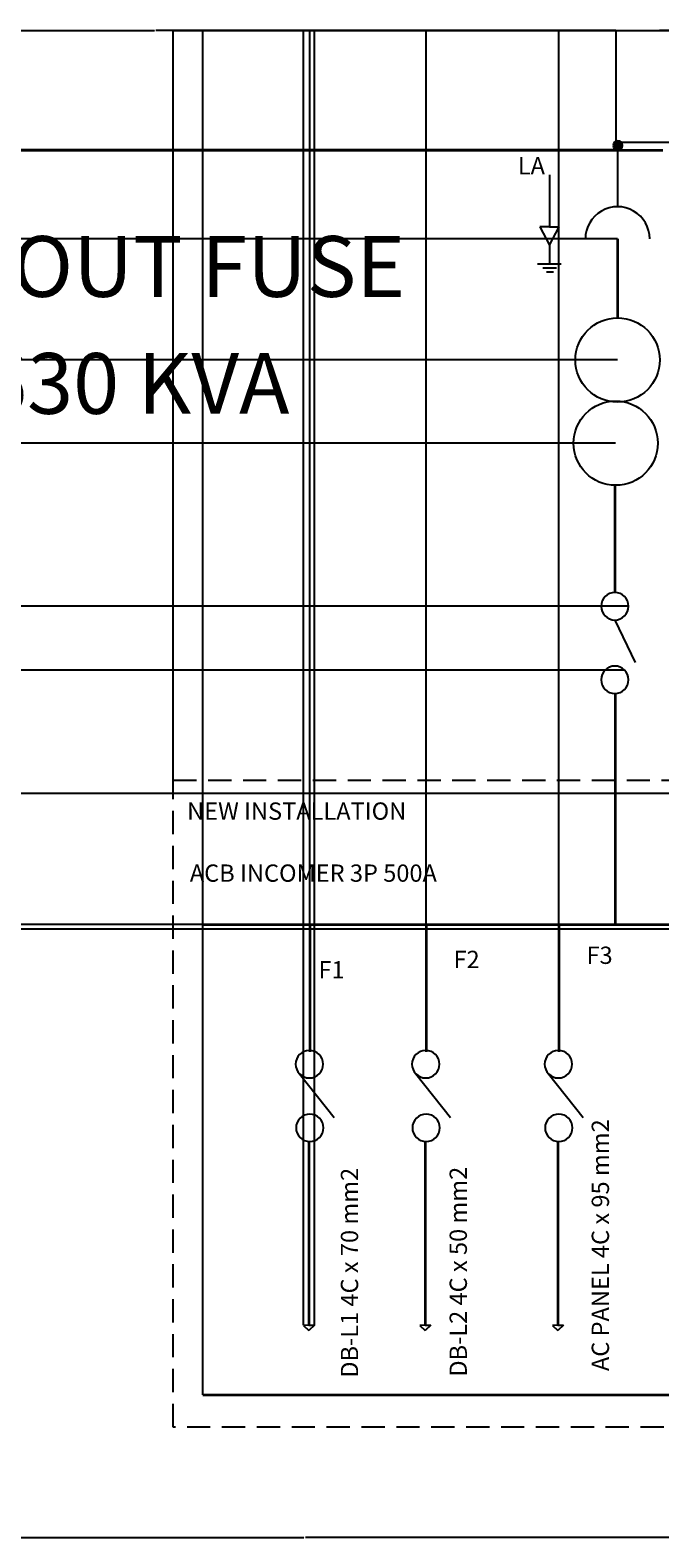
# Model space of a CAD drawing. Units: millimetres. Extents: x 1832 to 3146, y 927 to 1751.
# Tile 3 of 4: x 2339 to 2683, y 927 to 1751. Entities that reach past the tile are written whole.
import ezdxf

# ---------------------------------------------------------------- set-up
doc = ezdxf.new("R2010")
doc.units = ezdxf.units.MM
doc.header["$MEASUREMENT"] = 0
doc.linetypes.add('DASHED', pattern=[19.05, 12.7, -6.35])
doc.layers.get('0').update_dxf_attribs({"color": 2, "lineweight": 35})
doc.layers.get('0').transparency = 0.01
for name, color, linetype, lineweight in [('A-ANNO-DIMS', 2, 'Continuous', 18), ('E-ANNO-TEXT', 7, 'Continuous', 18), ('E-POWR-EQPM', 2, 'Continuous', 25), ('E-POWR-PNLS', 3, 'DASHED', 25), ('E-POWR-WIRE', 7, 'Continuous', 35)]:
    doc.layers.add(name, color=color, linetype=linetype, lineweight=lineweight)
doc.styles.get("Standard").update_dxf_attribs({"font": 'arial.ttf'})
doc.dimstyles.get("Standard").update_dxf_attribs({"dimtxt": 0.18, "dimasz": 0.18, "dimexe": 0.18, "dimexo": 0.0625, "dimgap": 0.09, "dimtad": 0, "dimtih": 1, "dimtoh": 1, "dimdec": 4, "dimzin": 0, "dimdsep": 46, "dimtxsty": 'Standard', "dimcen": 0.09, "dimadec": 0, "dimazin": 0, "dimtfac": 1, "dimtdec": 4, "dimtofl": 0, "dimtmove": 0, "dimatfit": 3, "dimfxl": 1, "dimtolj": 1, "dimtzin": 0, "dimarcsym": 0})

# ---------------------------------------------------------------- blocks, each defined once
blk = doc.blocks.new('CB-FEEDER')
blk.add_line((1982.97, 1178.23), (2001.83, 1154.39))
for points in [[(1980.83, 1183.48, 1), (1995.83, 1183.48, 1)], [(1981.05, 1148.75, 1), (1996.05, 1148.75, 1)]]:
    blk.add_lwpolyline(points, format="xyb", close=True)
blk = doc.blocks.new('CB-INCOMER')
blk.add_line((2155.16, 1426.14), (2166.26, 1402.88))
for points in [[(2147.67, 1433.64, 1), (2162.67, 1433.64, 1)], [(2147.67, 1393.5, 1), (2162.67, 1393.5, 1)]]:
    blk.add_lwpolyline(points, format="xyb", close=True)
blk = doc.blocks.new('CABLE-ARROW')
for p, q in [((1988.1, 1040.89), (1985.1, 1040.84)), ((1985.1, 1040.84), (1988.1, 1038.05)), ((1988.1, 1040.89), (1991.1, 1040.89)), ((1991.1, 1040.89), (1988.1, 1038.05))]:
    blk.add_line(p, q)
blk = doc.blocks.new('LIGHTNING-ARRESTER')
for p, q in [((2119.54, 1669.38), (2119.54, 1640.82)), ((2119.54, 1640.82), (2114.27, 1640.82)), ((2114.27, 1640.82), (2119.54, 1630.9)), ((2119.54, 1640.82), (2124.8, 1640.82)), ((2119.54, 1630.9), (2124.8, 1640.82)), ((2119.54, 1630.9), (2119.54, 1620.77)), ((2112.86, 1620.77), (2125.9, 1620.77)), ((2115.79, 1618.51), (2123.28, 1618.51)), ((2117.89, 1616.41), (2121.66, 1616.41))]:
    blk.add_line(p, q)
blk = doc.blocks.new('DROPOUT-FUSE')
h = blk.add_hatch(color=256)
h.dxf.hatch_style = 1
h.paths.add_polyline_path([(2154.3, 1685.32), (2159.3, 1685.32, 1)])
h.paths.add_polyline_path([(2159.3, 1685.32), (2154.3, 1685.32, 1)])
blk.add_line((2156.63, 1682.82), (2156.63, 1651.9))
blk.add_lwpolyline([(2154.3, 1685.32, 1), (2159.3, 1685.32, 1)], format="xyb", close=True)
blk.add_arc((2156.63, 1634.33), 17.57, 359.97103, 180.02897)
blk = doc.blocks.new('TRANSFORMER')
for centre in [(2156.63, 1568.17), (2155.63, 1522.72)]:
    blk.add_circle(centre, 23.01)
blk = doc.blocks.new('*D9')
at = {"layer": 'A-ANNO-DIMS', "color": 0, "lineweight": -2, "transparency": 16777216}
for p, q in [((1892.94, 1002.86), (1892.94, 927.26)), ((3085.33, 987.73), (3085.33, 927.26)), ((1893.12, 927.44), (2488.68, 927.44)), ((3085.15, 927.44), (2489.59, 927.44))]:
    blk.add_line(p, q, dxfattribs=at)
at = {"layer": 'A-ANNO-DIMS', "color": 0, "lineweight": 35, "transparency": 16777216}
for points in [[(1893.12, 927.47), (1893.12, 927.41), (1892.94, 927.44)], [(3085.15, 927.47), (3085.15, 927.41), (3085.33, 927.44)]]:
    blk.add_solid(points, dxfattribs=at)
at = {"layer": 'Defpoints', "color": 0, "lineweight": 35, "transparency": 16777216}
for p in [(1892.94, 1002.93), (3085.33, 987.79), (3085.33, 927.44)]:
    blk.add_point(p, dxfattribs=at)
at = {"layer": 'A-ANNO-DIMS', "color": 0, "transparency": 16777216, "insert": (2489.13, 927.44), "char_height": 0.18, "attachment_point": 5}
blk.add_mtext('\\A1;1192.4', dxfattribs=at)
blk = doc.blocks.new('*D10')
at = {"layer": 'A-ANNO-DIMS', "color": 0, "lineweight": -2, "transparency": 16777216}
for p, q in [((2658.48, 1689.58), (3145.86, 1689.58)), ((3145.68, 1689.4), (3145.68, 1338.87)), ((3145.68, 987.97), (3145.68, 1338.5)), ((3085.39, 987.79), (3145.86, 987.79))]:
    blk.add_line(p, q, dxfattribs=at)
at = {"layer": 'A-ANNO-DIMS', "color": 0, "lineweight": 35, "transparency": 16777216}
for points in [[(3145.65, 1689.4), (3145.71, 1689.4), (3145.68, 1689.58)], [(3145.65, 987.97), (3145.71, 987.97), (3145.68, 987.79)]]:
    blk.add_solid(points, dxfattribs=at)
at = {"layer": 'Defpoints', "color": 0, "lineweight": 35, "transparency": 16777216}
for p in [(2658.42, 1689.58), (3145.68, 1689.58), (3085.33, 987.79)]:
    blk.add_point(p, dxfattribs=at)
at = {"layer": 'A-ANNO-DIMS', "color": 0, "transparency": 16777216, "insert": (3145.68, 1338.68), "char_height": 0.18, "attachment_point": 5}
blk.add_mtext('\\A1;701.8', dxfattribs=at)
blk = doc.blocks.new('*D16')
at = {"layer": 'A-ANNO-DIMS', "color": 0, "lineweight": -2, "transparency": 16777216}
for p, q in [((2491.94, 1262.43), (2491.94, 1750.84)), ((2492.12, 1750.66), (2523.31, 1750.66)), ((2555.29, 1750.66), (2524.1, 1750.66)), ((2555.47, 1262.43), (2555.47, 1750.84))]:
    blk.add_line(p, q, dxfattribs=at)
at = {"layer": 'A-ANNO-DIMS', "color": 0, "lineweight": 35, "transparency": 16777216}
for points in [[(2492.12, 1750.69), (2492.12, 1750.63), (2491.94, 1750.66)], [(2555.29, 1750.69), (2555.29, 1750.63), (2555.47, 1750.66)]]:
    blk.add_solid(points, dxfattribs=at)
at = {"layer": 'Defpoints', "color": 0, "lineweight": 35, "transparency": 16777216}
for p in [(2555.47, 1750.66), (2491.94, 1262.37), (2555.47, 1262.37)]:
    blk.add_point(p, dxfattribs=at)
at = {"layer": 'A-ANNO-DIMS', "color": 0, "transparency": 16777216, "insert": (2523.7, 1750.66), "char_height": 0.18, "attachment_point": 5}
blk.add_mtext('\\A1;63.53', dxfattribs=at)
blk = doc.blocks.new('*D17')
at = {"layer": 'A-ANNO-DIMS', "color": 0, "lineweight": -2, "transparency": 16777216}
for p, q in [((2555.47, 1262.43), (2555.47, 1750.84)), ((2555.65, 1750.66), (2591.3, 1750.66)), ((2627.74, 1750.66), (2592.09, 1750.66)), ((2627.92, 1262.43), (2627.92, 1750.84))]:
    blk.add_line(p, q, dxfattribs=at)
at = {"layer": 'A-ANNO-DIMS', "color": 0, "lineweight": 35, "transparency": 16777216}
for points in [[(2555.65, 1750.69), (2555.65, 1750.63), (2555.47, 1750.66)], [(2627.74, 1750.69), (2627.74, 1750.63), (2627.92, 1750.66)]]:
    blk.add_solid(points, dxfattribs=at)
at = {"layer": 'Defpoints', "color": 0, "lineweight": 35, "transparency": 16777216}
for p in [(2627.92, 1750.66), (2555.47, 1262.37), (2627.92, 1262.37)]:
    blk.add_point(p, dxfattribs=at)
at = {"layer": 'A-ANNO-DIMS', "color": 0, "transparency": 16777216, "insert": (2591.69, 1750.66), "char_height": 0.18, "attachment_point": 5}
blk.add_mtext('\\A1;72.45', dxfattribs=at)
blk = doc.blocks.new('*D18')
at = {"layer": 'A-ANNO-DIMS', "color": 0, "lineweight": -2, "transparency": 16777216}
for p, q in [((2627.92, 1262.43), (2627.92, 1750.84)), ((2628.1, 1750.66), (2682.1, 1750.66)), ((2737.01, 1750.66), (2683.01, 1750.66)), ((2737.19, 1262.43), (2737.19, 1750.84))]:
    blk.add_line(p, q, dxfattribs=at)
at = {"layer": 'A-ANNO-DIMS', "color": 0, "lineweight": 35, "transparency": 16777216}
for points in [[(2628.1, 1750.69), (2628.1, 1750.63), (2627.92, 1750.66)], [(2737.01, 1750.69), (2737.01, 1750.63), (2737.19, 1750.66)]]:
    blk.add_solid(points, dxfattribs=at)
at = {"layer": 'Defpoints', "color": 0, "lineweight": 35, "transparency": 16777216}
for p in [(2737.19, 1750.66), (2627.92, 1262.37), (2737.19, 1262.37)]:
    blk.add_point(p, dxfattribs=at)
at = {"layer": 'A-ANNO-DIMS', "color": 0, "transparency": 16777216, "insert": (2682.56, 1750.66), "char_height": 0.18, "attachment_point": 5}
blk.add_mtext('\\A1;109.27', dxfattribs=at)
blk = doc.blocks.new('*D21')
at = {"layer": 'A-ANNO-DIMS', "color": 0, "lineweight": -2, "transparency": 16777216}
for p, q in [((2155.83, 1687.68), (2155.83, 1750.84)), ((2156.01, 1750.66), (2407.13, 1750.66)), ((2659.03, 1750.66), (2407.91, 1750.66)), ((2659.21, 1690.18), (2659.21, 1750.84))]:
    blk.add_line(p, q, dxfattribs=at)
at = {"layer": 'A-ANNO-DIMS', "color": 0, "lineweight": 35, "transparency": 16777216}
for points in [[(2156.01, 1750.69), (2156.01, 1750.63), (2155.83, 1750.66)], [(2659.03, 1750.69), (2659.03, 1750.63), (2659.21, 1750.66)]]:
    blk.add_solid(points, dxfattribs=at)
at = {"layer": 'Defpoints', "color": 0, "lineweight": 35, "transparency": 16777216}
for p in [(2659.21, 1750.66), (2659.21, 1690.11), (2155.83, 1687.62)]:
    blk.add_point(p, dxfattribs=at)
at = {"layer": 'A-ANNO-DIMS', "color": 0, "transparency": 16777216, "insert": (2407.52, 1750.66), "char_height": 0.18, "attachment_point": 5}
blk.add_mtext('\\A1;503.4', dxfattribs=at)
blk = doc.blocks.new('*D26')
at = {"layer": 'A-ANNO-DIMS', "color": 0, "lineweight": -2, "transparency": 16777216}
for p, q in [((2417.38, 1341.25), (2417.38, 1750.84)), ((2417.56, 1750.66), (2750.89, 1750.66)), ((3085.15, 1750.66), (2751.82, 1750.66)), ((3085.33, 1341.25), (3085.33, 1750.84))]:
    blk.add_line(p, q, dxfattribs=at)
at = {"layer": 'A-ANNO-DIMS', "color": 0, "lineweight": 35, "transparency": 16777216}
for points in [[(2417.56, 1750.69), (2417.56, 1750.63), (2417.38, 1750.66)], [(3085.15, 1750.69), (3085.15, 1750.63), (3085.33, 1750.66)]]:
    blk.add_solid(points, dxfattribs=at)
at = {"layer": 'Defpoints', "color": 0, "lineweight": 35, "transparency": 16777216}
for p in [(3085.33, 1750.66), (2417.38, 1341.19), (3085.33, 1341.19)]:
    blk.add_point(p, dxfattribs=at)
at = {"layer": 'A-ANNO-DIMS', "color": 0, "transparency": 16777216, "insert": (2751.35, 1750.66), "char_height": 0.18, "attachment_point": 5}
blk.add_mtext('\\A1;667.94', dxfattribs=at)
blk = doc.blocks.new('*D28')
at = {"layer": 'A-ANNO-DIMS', "color": 0, "lineweight": -2, "transparency": 16777216}
for p, q in [((2433.56, 1005.45), (2433.56, 1750.84)), ((2433.74, 1750.66), (2748.28, 1750.66)), ((3063.74, 1750.66), (2749.21, 1750.66)), ((3063.92, 1005.45), (3063.92, 1750.84))]:
    blk.add_line(p, q, dxfattribs=at)
at = {"layer": 'A-ANNO-DIMS', "color": 0, "lineweight": 35, "transparency": 16777216}
for points in [[(2433.74, 1750.69), (2433.74, 1750.63), (2433.56, 1750.66)], [(3063.74, 1750.69), (3063.74, 1750.63), (3063.92, 1750.66)]]:
    blk.add_solid(points, dxfattribs=at)
at = {"layer": 'Defpoints', "color": 0, "lineweight": 35, "transparency": 16777216}
for p in [(3063.92, 1750.66), (2433.56, 1005.39), (3063.92, 1005.39)]:
    blk.add_point(p, dxfattribs=at)
at = {"layer": 'A-ANNO-DIMS', "color": 0, "transparency": 16777216, "insert": (2748.74, 1750.66), "char_height": 0.18, "attachment_point": 5}
blk.add_mtext('\\A1;630.36', dxfattribs=at)
blk = doc.blocks.new('*D30')
at = {"layer": 'A-ANNO-DIMS', "color": 0, "lineweight": -2, "transparency": 16777216}
for p, q in [((2433.56, 1262.43), (2433.56, 1750.84)), ((2433.74, 1750.66), (2462.36, 1750.66)), ((2491.76, 1750.66), (2463.14, 1750.66)), ((2491.94, 1262.43), (2491.94, 1750.84))]:
    blk.add_line(p, q, dxfattribs=at)
at = {"layer": 'A-ANNO-DIMS', "color": 0, "lineweight": 35, "transparency": 16777216}
for points in [[(2433.74, 1750.69), (2433.74, 1750.63), (2433.56, 1750.66)], [(2491.76, 1750.69), (2491.76, 1750.63), (2491.94, 1750.66)]]:
    blk.add_solid(points, dxfattribs=at)
at = {"layer": 'Defpoints', "color": 0, "lineweight": 35, "transparency": 16777216}
for p in [(2491.94, 1750.66), (2433.56, 1262.37), (2491.94, 1262.37)]:
    blk.add_point(p, dxfattribs=at)
at = {"layer": 'A-ANNO-DIMS', "color": 0, "transparency": 16777216, "insert": (2462.75, 1750.66), "char_height": 0.18, "attachment_point": 5}
blk.add_mtext('\\A1;58.37', dxfattribs=at)
blk = doc.blocks.new('*D33')
at = {"layer": 'A-ANNO-DIMS', "color": 0, "lineweight": -2, "transparency": 16777216}
for p, q in [((2659.21, 1685.57), (2659.21, 1750.84)), ((2659.39, 1750.66), (2813.63, 1750.66)), ((2968.8, 1750.66), (2814.56, 1750.66)), ((2968.98, 1685.38), (2968.98, 1750.84))]:
    blk.add_line(p, q, dxfattribs=at)
at = {"layer": 'A-ANNO-DIMS', "color": 0, "lineweight": 35, "transparency": 16777216}
for points in [[(2659.39, 1750.69), (2659.39, 1750.63), (2659.21, 1750.66)], [(2968.8, 1750.69), (2968.8, 1750.63), (2968.98, 1750.66)]]:
    blk.add_solid(points, dxfattribs=at)
at = {"layer": 'Defpoints', "color": 0, "lineweight": 35, "transparency": 16777216}
for p in [(2968.98, 1750.66), (2659.21, 1685.51), (2968.98, 1685.32)]:
    blk.add_point(p, dxfattribs=at)
at = {"layer": 'A-ANNO-DIMS', "color": 0, "transparency": 16777216, "insert": (2814.1, 1750.66), "char_height": 0.18, "attachment_point": 5}
blk.add_mtext('\\A1;309.76', dxfattribs=at)
blk = doc.blocks.new('*D47')
at = {"layer": 'A-ANNO-DIMS', "color": 0, "lineweight": -2, "transparency": 16777216}
for p, q in [((2330.79, 1334.1), (3145.86, 1334.1)), ((3145.68, 1333.92), (3145.68, 1297.17)), ((3145.68, 1260.06), (3145.68, 1296.81)), ((2311.47, 1259.88), (3145.86, 1259.88))]:
    blk.add_line(p, q, dxfattribs=at)
at = {"layer": 'A-ANNO-DIMS', "color": 0, "lineweight": 35, "transparency": 16777216}
for points in [[(3145.65, 1333.92), (3145.71, 1333.92), (3145.68, 1334.1)], [(3145.65, 1260.06), (3145.71, 1260.06), (3145.68, 1259.88)]]:
    blk.add_solid(points, dxfattribs=at)
at = {"layer": 'Defpoints', "color": 0, "lineweight": 35, "transparency": 16777216}
for p in [(2330.73, 1334.1), (2311.41, 1259.88), (3145.68, 1259.88)]:
    blk.add_point(p, dxfattribs=at)
at = {"layer": 'A-ANNO-DIMS', "color": 0, "transparency": 16777216, "insert": (3145.68, 1296.99), "char_height": 0.18, "attachment_point": 5}
blk.add_mtext('\\A1;74.22', dxfattribs=at)
blk = doc.blocks.new('*D50')
at = {"layer": 'A-ANNO-DIMS', "color": 0, "lineweight": -2, "transparency": 16777216}
for p, q in [((2663.8, 1401.3), (1832.41, 1401.3)), ((1832.59, 1401.12), (1832.59, 1332.02)), ((1832.59, 1262.55), (1832.59, 1331.65)), ((2658.71, 1262.37), (1832.41, 1262.37))]:
    blk.add_line(p, q, dxfattribs=at)
at = {"layer": 'A-ANNO-DIMS', "color": 0, "lineweight": 35, "transparency": 16777216}
for points in [[(1832.56, 1401.12), (1832.62, 1401.12), (1832.59, 1401.3)], [(1832.56, 1262.55), (1832.62, 1262.55), (1832.59, 1262.37)]]:
    blk.add_solid(points, dxfattribs=at)
at = {"layer": 'Defpoints', "color": 0, "lineweight": 35, "transparency": 16777216}
for p in [(1832.59, 1401.3), (2663.86, 1401.3), (2658.78, 1262.37)]:
    blk.add_point(p, dxfattribs=at)
at = {"layer": 'A-ANNO-DIMS', "color": 0, "transparency": 16777216, "insert": (1832.59, 1331.83), "char_height": 0.18, "attachment_point": 5}
blk.add_mtext('\\A1;138.92', dxfattribs=at)
blk = doc.blocks.new('*D51')
at = {"layer": 'A-ANNO-DIMS', "color": 0, "lineweight": -2, "transparency": 16777216}
for p, q in [((2665.99, 1436.13), (1832.41, 1436.13)), ((1832.59, 1435.95), (1832.59, 1418.9)), ((1832.59, 1401.48), (1832.59, 1418.53)), ((2663.8, 1401.3), (1832.41, 1401.3))]:
    blk.add_line(p, q, dxfattribs=at)
at = {"layer": 'A-ANNO-DIMS', "color": 0, "lineweight": 35, "transparency": 16777216}
for points in [[(1832.56, 1435.95), (1832.62, 1435.95), (1832.59, 1436.13)], [(1832.56, 1401.48), (1832.62, 1401.48), (1832.59, 1401.3)]]:
    blk.add_solid(points, dxfattribs=at)
at = {"layer": 'Defpoints', "color": 0, "lineweight": 35, "transparency": 16777216}
for p in [(1832.59, 1436.13), (2666.06, 1436.13), (2663.86, 1401.3)]:
    blk.add_point(p, dxfattribs=at)
at = {"layer": 'A-ANNO-DIMS', "color": 0, "transparency": 16777216, "insert": (1832.59, 1418.71), "char_height": 0.18, "attachment_point": 5}
blk.add_mtext('\\A1;34.83', dxfattribs=at)
blk = doc.blocks.new('*D52')
at = {"layer": 'A-ANNO-DIMS', "color": 0, "lineweight": -2, "transparency": 16777216}
for p, q in [((2658.96, 1525.22), (1832.41, 1525.22)), ((1832.59, 1525.04), (1832.59, 1480.86)), ((1832.59, 1436.31), (1832.59, 1480.49)), ((2665.99, 1436.13), (1832.41, 1436.13))]:
    blk.add_line(p, q, dxfattribs=at)
at = {"layer": 'A-ANNO-DIMS', "color": 0, "lineweight": 35, "transparency": 16777216}
for points in [[(1832.56, 1525.04), (1832.62, 1525.04), (1832.59, 1525.22)], [(1832.56, 1436.31), (1832.62, 1436.31), (1832.59, 1436.13)]]:
    blk.add_solid(points, dxfattribs=at)
at = {"layer": 'Defpoints', "color": 0, "lineweight": 35, "transparency": 16777216}
for p in [(1832.59, 1525.22), (2659.02, 1525.22), (2666.06, 1436.13)]:
    blk.add_point(p, dxfattribs=at)
at = {"layer": 'A-ANNO-DIMS', "color": 0, "transparency": 16777216, "insert": (1832.59, 1480.67), "char_height": 0.18, "attachment_point": 5}
blk.add_mtext('\\A1;89.09', dxfattribs=at)
blk = doc.blocks.new('*D53')
at = {"layer": 'A-ANNO-DIMS', "color": 0, "lineweight": -2, "transparency": 16777216}
for p, q in [((2659.96, 1570.67), (1832.41, 1570.67)), ((1832.59, 1570.49), (1832.59, 1548.12)), ((1832.59, 1525.4), (1832.59, 1547.76)), ((2658.96, 1525.22), (1832.41, 1525.22))]:
    blk.add_line(p, q, dxfattribs=at)
at = {"layer": 'A-ANNO-DIMS', "color": 0, "lineweight": 35, "transparency": 16777216}
for points in [[(1832.56, 1570.49), (1832.62, 1570.49), (1832.59, 1570.67)], [(1832.56, 1525.4), (1832.62, 1525.4), (1832.59, 1525.22)]]:
    blk.add_solid(points, dxfattribs=at)
at = {"layer": 'Defpoints', "color": 0, "lineweight": 35, "transparency": 16777216}
for p in [(1832.59, 1570.67), (2660.02, 1570.67), (2659.02, 1525.22)]:
    blk.add_point(p, dxfattribs=at)
at = {"layer": 'A-ANNO-DIMS', "color": 0, "transparency": 16777216, "insert": (1832.59, 1547.94), "char_height": 0.18, "attachment_point": 5}
blk.add_mtext('\\A1;45.45', dxfattribs=at)
blk = doc.blocks.new('*D54')
at = {"layer": 'A-ANNO-DIMS', "color": 0, "lineweight": -2, "transparency": 16777216}
for p, q in [((2659.96, 1636.83), (1832.41, 1636.83)), ((1832.59, 1636.65), (1832.59, 1603.93)), ((1832.59, 1570.85), (1832.59, 1603.56)), ((2659.96, 1570.67), (1832.41, 1570.67))]:
    blk.add_line(p, q, dxfattribs=at)
at = {"layer": 'A-ANNO-DIMS', "color": 0, "lineweight": 35, "transparency": 16777216}
for points in [[(1832.56, 1636.65), (1832.62, 1636.65), (1832.59, 1636.83)], [(1832.56, 1570.85), (1832.62, 1570.85), (1832.59, 1570.67)]]:
    blk.add_solid(points, dxfattribs=at)
at = {"layer": 'Defpoints', "color": 0, "lineweight": 35, "transparency": 16777216}
for p in [(1832.59, 1636.83), (2660.02, 1636.83), (2660.02, 1570.67)]:
    blk.add_point(p, dxfattribs=at)
at = {"layer": 'A-ANNO-DIMS', "color": 0, "transparency": 16777216, "insert": (1832.59, 1603.75), "char_height": 0.18, "attachment_point": 5}
blk.add_mtext('\\A1;66.16', dxfattribs=at)
blk = doc.blocks.new('*D55')
at = {"layer": 'A-ANNO-DIMS', "color": 0, "lineweight": -2, "transparency": 16777216}
for p, q in [((2659.15, 1685.51), (1832.41, 1685.51)), ((1832.59, 1685.33), (1832.59, 1661.35)), ((1832.59, 1637.01), (1832.59, 1660.98)), ((2659.96, 1636.83), (1832.41, 1636.83))]:
    blk.add_line(p, q, dxfattribs=at)
at = {"layer": 'A-ANNO-DIMS', "color": 0, "lineweight": 35, "transparency": 16777216}
for points in [[(1832.56, 1685.33), (1832.62, 1685.33), (1832.59, 1685.51)], [(1832.56, 1637.01), (1832.62, 1637.01), (1832.59, 1636.83)]]:
    blk.add_solid(points, dxfattribs=at)
at = {"layer": 'Defpoints', "color": 0, "lineweight": 35, "transparency": 16777216}
for p in [(1832.59, 1685.51), (2659.21, 1685.51), (2660.02, 1636.83)]:
    blk.add_point(p, dxfattribs=at)
at = {"layer": 'A-ANNO-DIMS', "color": 0, "transparency": 16777216, "insert": (1832.59, 1661.17), "char_height": 0.18, "attachment_point": 5}
blk.add_mtext('\\A1;48.68', dxfattribs=at)
blk = doc.blocks.new('*D56')
at = {"layer": 'A-ANNO-DIMS', "color": 0, "lineweight": -2, "transparency": 16777216}
for p, q in [((2488.49, 1043.39), (2488.49, 1750.84)), ((2488.67, 1750.66), (2491.16, 1750.66)), ((2494.31, 1750.66), (2491.81, 1750.66)), ((2494.49, 1043.45), (2494.49, 1750.84))]:
    blk.add_line(p, q, dxfattribs=at)
at = {"layer": 'A-ANNO-DIMS', "color": 0, "lineweight": 35, "transparency": 16777216}
for points in [[(2488.67, 1750.69), (2488.67, 1750.63), (2488.49, 1750.66)], [(2494.31, 1750.69), (2494.31, 1750.63), (2494.49, 1750.66)]]:
    blk.add_solid(points, dxfattribs=at)
at = {"layer": 'Defpoints', "color": 0, "lineweight": 35, "transparency": 16777216}
for p in [(2494.49, 1750.66), (2488.49, 1043.33), (2494.49, 1043.39)]:
    blk.add_point(p, dxfattribs=at)
at = {"layer": 'A-ANNO-DIMS', "color": 0, "transparency": 16777216, "insert": (2491.49, 1750.66), "char_height": 0.18, "attachment_point": 5}
blk.add_mtext('\\A1;6.00', dxfattribs=at)

msp = doc.modelspace()

# ---------------------------------------------------------------- linework, layer by layer
at = {"layer": 'E-POWR-PNLS'}
msp.add_lwpolyline([(2417.3834, 1341.189), (3085.3254, 1341.189), (3085.3254, 987.7892), (2417.3834, 987.7892)], close=True, dxfattribs=at)
at = {"layer": 'E-POWR-WIRE'}
for p, q in [((2063.171, 1685.3164), (2684.8145, 1685.3164)), ((2660.0216, 1636.8256), (2660.0216, 1593.6756)), ((2658.5568, 1502.2129), (2658.5568, 1443.6305)), ((2658.7774, 1388.4972), (2658.7774, 1262.3723)), ((2433.5628, 1262.3723), (2814.7999, 1262.3723)), ((2491.9363, 1262.3723), (2491.9363, 1192.7373)), ((2555.4686, 1262.3723), (2555.4686, 1192.7373)), ((2627.9202, 1262.3723), (2627.9202, 1192.7373)), ((2491.487, 1143.7615), (2491.487, 1043.3883)), ((2555.0192, 1143.7615), (2555.0192, 1043.3883)), ((2627.4708, 1143.7615), (2627.4708, 1043.3883)), ((2433.5628, 1005.3868), (3063.9193, 1005.3868))]:
    msp.add_line(p, q, dxfattribs=at)

# ---------------------------------------------------------------- block references
at = {"layer": 'E-POWR-EQPM'}
for name, p in [('DROPOUT-FUSE', (503.3881, 2.4945)), ('LIGHTNING-ARRESTER', (503.3881, 2.4945)), ('TRANSFORMER', (503.3881, 2.4945)), ('CB-INCOMER', (503.3881, 2.4945)), ('CB-FEEDER', (503.3881, 2.4945)), ('CB-FEEDER', (566.9204, 2.4945)), ('CB-FEEDER', (639.3719, 2.4945)), ('CABLE-ARROW', (503.3881, 2.4945)), ('CABLE-ARROW', (566.9204, 2.4945)), ('CABLE-ARROW', (639.3719, 2.4945))]:
    msp.add_blockref(name, p, dxfattribs=at)

# ---------------------------------------------------------------- texts
at = {"layer": 'E-ANNO-TEXT'}
for s, height, p in [('LA', 9.44797, (2605.5428, 1672.0495)), ('DROP OUT FUSE', 33.205653, (2196.7504, 1605.1502)), ('TR-1 630 KVA', 33.205653, (2205.5164, 1541.2551)), ('NEW INSTALLATION', 9.447971, (2424.9533, 1319.5245)), ('ACB INCOMER 3P 500A', 9.447971, (2426.4264, 1285.649)), ('F2', 9.44797, (2570.444, 1238.5031)), ('F3', 9.44797, (2643.0662, 1240.7706)), ('F1', 9.44797, (2496.6872, 1232.8345))]:
    msp.add_text(s, height=height, dxfattribs=at).set_placement(p)
for s, p in [('AC PANEL 4C x 95 mm2', (2655.3459, 1018.3546)), ('DB-L1 4C x 70 mm2', (2518.3528, 1014.7332)), ('DB-L2 4C x 50 mm2', (2577.7549, 1015.3239))]:
    msp.add_text(s, height=9.447971, rotation=90, dxfattribs=at).set_placement(p)

# ---------------------------------------------------------------- dimensions: what is measured, and where the dimension line sits
at = {"layer": 'A-ANNO-DIMS'}
for base, p1, p2, override, picture, middle in [((2659.2142, 1750.6609), (2155.8261, 1687.62), (2659.2142, 1690.1145), {"dimdec": 1, "dimlfac": 1, "dimrnd": 0, "dimzin": 0, "dimdsep": 46, "dimlunit": 2}, '*D21', (2407.5202, 1750.6609)), ((3085.3254, 1750.6609), (2417.3834, 1341.189), (3085.3254, 1341.189), {"dimdec": 2, "dimlfac": 1, "dimrnd": 0, "dimzin": 0, "dimdsep": 46, "dimlunit": 2}, '*D26', (2751.3544, 1750.6609)), ((3063.9193, 1750.6609), (2433.5628, 1005.3868), (3063.9193, 1005.3868), {"dimdec": 2, "dimlfac": 1, "dimrnd": 0, "dimzin": 0, "dimdsep": 46, "dimlunit": 2}, '*D28', (2748.741, 1750.6609)), ((2491.9363, 1750.6609), (2433.5628, 1262.3723), (2491.9363, 1262.3723), {"dimdec": 2, "dimlfac": 1, "dimrnd": 0, "dimzin": 0, "dimdsep": 46, "dimlunit": 2}, '*D30', (2462.7496, 1750.6609)), ((2494.487, 1750.6609), (2488.4875, 1043.3308), (2494.487, 1043.3883), {"dimdec": 2, "dimlfac": 1, "dimrnd": 0, "dimzin": 0, "dimdsep": 46, "dimlunit": 2}, '*D56', (2491.4872, 1750.6609)), ((2555.4686, 1750.6609), (2491.9363, 1262.3723), (2555.4686, 1262.3723), {"dimdec": 2, "dimlfac": 1, "dimrnd": 0, "dimzin": 0, "dimdsep": 46, "dimlunit": 2}, '*D16', (2523.7025, 1750.6609)), ((2627.9202, 1750.6609), (2555.4686, 1262.3723), (2627.9202, 1262.3723), {"dimdec": 2, "dimlfac": 1, "dimrnd": 0, "dimzin": 0, "dimdsep": 46, "dimlunit": 2}, '*D17', (2591.6944, 1750.6609)), ((2737.1914, 1750.6609), (2627.9202, 1262.3723), (2737.1914, 1262.3723), {"dimdec": 2, "dimlfac": 1, "dimrnd": 0, "dimzin": 0, "dimdsep": 46, "dimlunit": 2}, '*D18', (2682.5558, 1750.6609)), ((2968.9766, 1750.6609), (2659.2142, 1685.5074), (2968.9766, 1685.3164), {"dimdec": 2, "dimlfac": 1, "dimrnd": 0, "dimzin": 0, "dimdsep": 46, "dimlunit": 2}, '*D33', (2814.0954, 1750.6609)), ((3085.3254, 927.4392), (1892.9387, 1002.9254), (3085.3254, 987.7892), {"dimdec": 1, "dimlfac": 1, "dimrnd": 0, "dimzin": 0, "dimdsep": 46, "dimlunit": 2}, '*D9', (2489.1321, 927.4392))]:
    dim = msp.add_linear_dim(base=base, p1=p1, p2=p2, dimstyle='Standard', override=override, dxfattribs=at)
    dim.commit()
    dim.dimension.update_dxf_attribs({"geometry": picture, "text_midpoint": middle})
for base, p1, p2, override, picture, middle in [((3145.6754, 1689.5787), (3085.3254, 987.7892), (2658.4196, 1689.5787), {"dimdec": 1, "dimlfac": 1, "dimrnd": 0, "dimzin": 0, "dimdsep": 46, "dimlunit": 2}, '*D10', (3145.6754, 1338.6839)), ((1832.5887, 1685.5074), (2660.0216, 1636.8256), (2659.2142, 1685.5074), {"dimdec": 2, "dimlfac": 1, "dimrnd": 0, "dimzin": 0, "dimdsep": 46, "dimlunit": 2}, '*D55', (1832.5887, 1661.1665)), ((1832.5887, 1636.8256), (2660.0216, 1570.6655), (2660.0216, 1636.8256), {"dimdec": 2, "dimlfac": 1, "dimrnd": 0, "dimzin": 0, "dimdsep": 46, "dimlunit": 2}, '*D54', (1832.5887, 1603.7456)), ((1832.5887, 1570.6655), (2659.0206, 1525.2183), (2660.0216, 1570.6655), {"dimdec": 2, "dimlfac": 1, "dimrnd": 0, "dimzin": 0, "dimdsep": 46, "dimlunit": 2}, '*D53', (1832.5887, 1547.9419)), ((1832.5887, 1525.2183), (2666.0568, 1436.1305), (2659.0206, 1525.2183), {"dimdec": 2, "dimlfac": 1, "dimrnd": 0, "dimzin": 0, "dimdsep": 46, "dimlunit": 2}, '*D52', (1832.5887, 1480.6744)), ((1832.5887, 1436.1305), (2663.8601, 1401.2973), (2666.0568, 1436.1305), {"dimdec": 2, "dimlfac": 1, "dimrnd": 0, "dimzin": 0, "dimdsep": 46, "dimlunit": 2}, '*D51', (1832.5887, 1418.7139)), ((1832.58868, 1401.29727), (2658.77741, 1262.37233), (2663.86014, 1401.29727), {"dimdec": 2, "dimlfac": 1, "dimrnd": 0, "dimzin": 0, "dimdsep": 46, "dimlunit": 2}, '*D50', (1832.58868, 1331.8348)), ((3145.6754, 1259.8778), (2330.7306, 1334.0963), (2311.4119, 1259.8778), {"dimdec": 2, "dimlfac": 1, "dimrnd": 0, "dimzin": 0, "dimdsep": 46, "dimlunit": 2}, '*D47', (3145.6754, 1296.9871))]:
    dim = msp.add_linear_dim(base=base, p1=p1, p2=p2, angle=90, dimstyle='Standard', override=override, dxfattribs=at)
    dim.commit()
    dim.dimension.update_dxf_attribs({"geometry": picture, "text_midpoint": middle})

doc.saveas('drawing.dxf')
